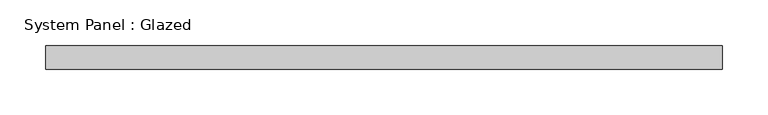
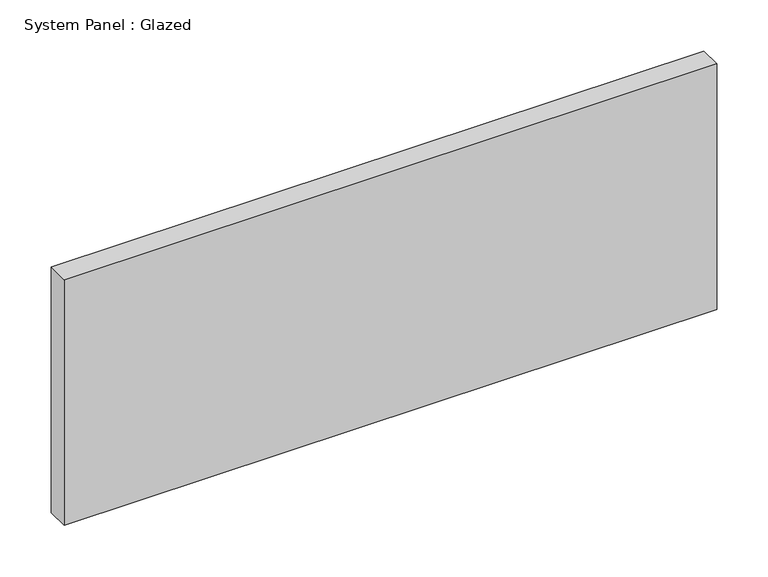
"""IFC4 building model written with IfcOpenShell, lengths in millimetres: plate geometry, System Panel : Glazed."""

from ifc_helpers import new_model, si_unit, origin, origin_with_axes, place, context, project, spatial, polyline, outline, extrude, source, transform, mapped, element, save


def system_panel_glazed_b4a359f9(model_context):
    return source(origin(), model_context, "Body", "SweptSolid", [
        extrude(outline(polyline([(369.22075, 19.05), (-369.22075, 19.05), (-369.22075, 44.45), (369.22075, 44.45), (369.22075, 19.05)])), origin_with_axes(), (0.0, 0.0, 1.0), 293.9415),
    ])


if __name__ == "__main__":
    model = new_model("IFC4")
    model_context = context("Model", 3, world=origin())
    ifc_project = project(units=[si_unit("LENGTHUNIT", "METRE", prefix="MILLI")], contexts=[model_context])
    site = spatial("IfcSite", under=ifc_project)
    building = spatial("IfcBuilding", under=site)
    placement = place(None, origin())
    system_panel_glazed_shape = system_panel_glazed_b4a359f9(model_context)
    element("IfcPlate", 1, ObjectType="System Panel : Glazed", at=placement, inside=building, context=model_context, shape_type="MappedRepresentation", body=[
        mapped(system_panel_glazed_shape, transform((0.0, 0.0, 0.0), x_axis=(1.0, 0.0, 0.0), y_axis=(0.0, 1.0, 0.0), z_axis=(0.0, 0.0, 1.0))),
    ])
    save(model, "model.ifc")

# Revit data of these elements
# Type "System Panel : Glazed"
#   Construction Type Id = "GSP4R"
#   Analytic Construction = "1/8 in Pilkington single glazing"
#   Visual Light Transmittance = 0.9
#   Solar Heat Gain Coefficient = 0.86
#   Heat Transfer Coefficient (U) = 1.18115 BTU/(h·ft²·°F)
#   Define Thermal Properties by = 1
# Element 1 (IfcPlate, "System Panel : Glazed")
#   Materials on its faces: "Glass"
# Materials
#   "Glass": class "Glass", colour RGB 0 128 192, transparency 0.75, Description = "Soda Lime Glass", Cost = 0
